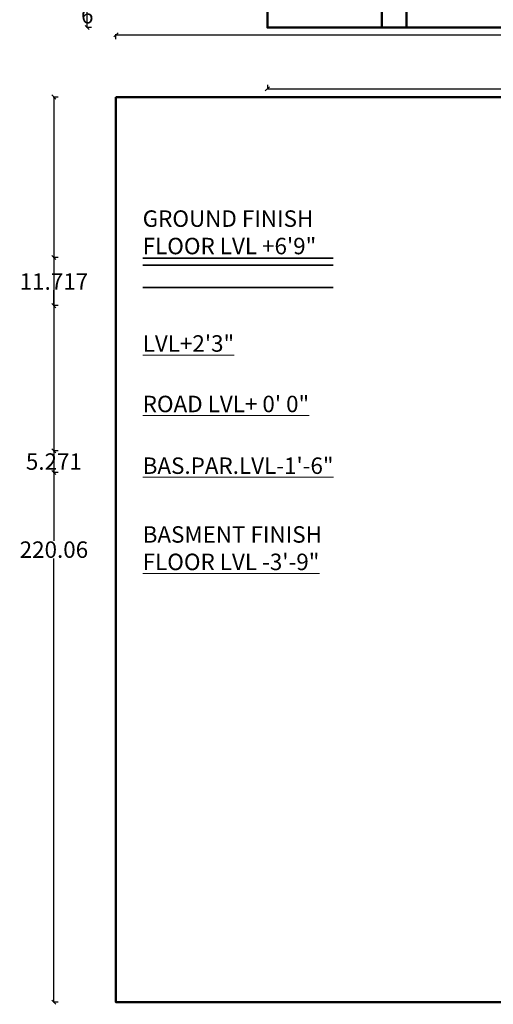
# Model space of a CAD drawing. Units: inches. Extents: x -60 to 284, y -245 to 257.
# Tile 1 of 10: x -60 to 55, y -228 to 12. Entities that reach past the tile are written whole.
import ezdxf

# ---------------------------------------------------------------- set-up
doc = ezdxf.new("R2010")
doc.units = ezdxf.units.IN
doc.header["$LTSCALE"] = 0.8
doc.header["$MEASUREMENT"] = 0
for name, color, linetype, lineweight in [('A-ANNO-DIMS', 2, 'Continuous', 18), ('A-ANNO-TEXT', 3, 'Continuous', 18), ('A-ANNO-TTLB', 7, 'Continuous', 50), ('A-SECT', 7, 'Continuous', 35), ('A-WALL', 7, 'Continuous', 50)]:
    doc.layers.add(name, color=color, linetype=linetype, lineweight=lineweight)
doc.styles.get("Standard").update_dxf_attribs({"font": 'arial.ttf'})
doc.dimstyles.get("Standard").update_dxf_attribs({"dimtxt": 4, "dimasz": 1, "dimexe": 0.18, "dimexo": 0.0625, "dimgap": 0.09, "dimtad": 0, "dimtih": 1, "dimtoh": 1, "dimzin": 0, "dimdsep": 46, "dimlunit": 4, "dimtxsty": 'Standard', "dimblk": 'OBLIQUE', "dimcen": 0.09, "dimadec": 0, "dimazin": 0, "dimtfac": 1, "dimtofl": 0, "dimtmove": 0, "dimatfit": 3, "dimfxl": 1, "dimfxlon": 1, "dimtolj": 1, "dimtzin": 0, "dimarcsym": 0})

# ---------------------------------------------------------------- blocks, each defined once
blk = doc.blocks.new('_Oblique')
at = {"color": 0, "linetype": 'ByBlock', "lineweight": -2}
blk.add_line((-0.5, -0.5), (0.5, 0.5), dxfattribs=at)
blk = doc.blocks.new('*D89')
at = {"layer": 'A-ANNO-DIMS', "color": 0, "lineweight": -2, "ltscale": 0.8, "transparency": 16777216}
for p, q in [((0.09, -4.23), (0.09, -5.41)), ((239.66, -4.23), (239.66, -5.41)), ((0.09, -5.23), (113, -5.23)), ((239.66, -5.23), (126.75, -5.23))]:
    blk.add_line(p, q, dxfattribs=at)
at = {"layer": 'Defpoints', "color": 0, "ltscale": 0.8, "transparency": 16777216}
for p in [(0.09, 9.67), (239.66, 9.67), (239.66, -5.23)]:
    blk.add_point(p, dxfattribs=at)
at = {"layer": 'A-ANNO-DIMS', "color": 0, "lineweight": -2, "ltscale": 0.8, "transparency": 16777216, "rotation": 180}
blk.add_blockref('_Oblique', (0.09, -5.23), dxfattribs=at)
at = {"layer": 'A-ANNO-DIMS', "color": 0, "lineweight": -2, "ltscale": 0.8, "transparency": 16777216}
blk.add_blockref('_Oblique', (239.66, -5.23), dxfattribs=at)
at = {"layer": 'A-ANNO-DIMS', "color": 0, "ltscale": 0.8, "transparency": 16777216, "insert": (119.88, -5.23), "char_height": 4, "attachment_point": 5}
blk.add_mtext('\\A1;239.6', dxfattribs=at)
blk = doc.blocks.new('*D90')
at = {"layer": 'A-ANNO-DIMS', "color": 0, "lineweight": -2, "ltscale": 0.8, "transparency": 16777216}
for p, q in [((-42.73, 122.67), (-43.91, 122.67)), ((-43.73, 122.67), (-43.73, 68.3)), ((-43.73, 9.67), (-43.73, 64.03)), ((-42.73, 9.67), (-43.91, 9.67))]:
    blk.add_line(p, q, dxfattribs=at)
at = {"layer": 'Defpoints', "color": 0, "ltscale": 0.8, "transparency": 16777216}
for p in [(-43.73, 122.67), (0.09, 122.67), (0.09, 9.67)]:
    blk.add_point(p, dxfattribs=at)
at = {"layer": 'A-ANNO-DIMS', "color": 0, "lineweight": -2, "ltscale": 0.8, "transparency": 16777216}
for p, rotation in [((-43.73, 122.67), 90), ((-43.73, 9.67), 270)]:
    blk.add_blockref('_Oblique', p, dxfattribs=dict(at, rotation=rotation))
at = {"layer": 'A-ANNO-DIMS', "color": 0, "ltscale": 0.8, "transparency": 16777216, "insert": (-43.73, 66.17), "char_height": 4, "attachment_point": 5}
blk.add_mtext('\\A1;113', dxfattribs=at)
blk = doc.blocks.new('*D101')
at = {"layer": 'A-ANNO-DIMS', "color": 0, "lineweight": -2, "ltscale": 0.8, "transparency": 16777216}
for p, q in [((-42.73, 15.67), (-43.91, 15.67)), ((-43.73, 15.67), (-43.73, 14.8)), ((-42.73, 9.67), (-43.91, 9.67)), ((-43.73, 9.67), (-43.73, 10.53))]:
    blk.add_line(p, q, dxfattribs=at)
at = {"layer": 'Defpoints', "color": 0, "ltscale": 0.8, "transparency": 16777216}
for p in [(-43.73, 15.67), (33.94, 15.67), (33.94, 9.67)]:
    blk.add_point(p, dxfattribs=at)
at = {"layer": 'A-ANNO-DIMS', "color": 0, "lineweight": -2, "ltscale": 0.8, "transparency": 16777216}
for p, rotation in [((-43.73, 15.67), 90), ((-43.73, 9.67), 270)]:
    blk.add_blockref('_Oblique', p, dxfattribs=dict(at, rotation=rotation))
at = {"layer": 'A-ANNO-DIMS', "color": 0, "ltscale": 0.8, "transparency": 16777216, "insert": (-43.73, 12.67), "char_height": 4, "attachment_point": 5}
blk.add_mtext('\\A1;6', dxfattribs=at)
blk = doc.blocks.new('*D106')
at = {"layer": 'A-ANNO-DIMS', "color": 0, "lineweight": -2, "ltscale": 0.8, "transparency": 16777216}
for p, q in [((-50.85, -93.21), (-52.03, -93.21)), ((-51.85, -93.21), (-51.85, -93.71)), ((-51.85, -98.48), (-51.85, -97.98)), ((-50.85, -98.48), (-52.03, -98.48))]:
    blk.add_line(p, q, dxfattribs=at)
at = {"layer": 'Defpoints', "color": 0, "ltscale": 0.8, "transparency": 16777216}
for p in [(67.01, -93.21), (-51.85, -98.48), (67.01, -98.48)]:
    blk.add_point(p, dxfattribs=at)
at = {"layer": 'A-ANNO-DIMS', "color": 0, "lineweight": -2, "ltscale": 0.8, "transparency": 16777216}
for p, rotation in [((-51.85, -93.21), 90), ((-51.85, -98.48), 270)]:
    blk.add_blockref('_Oblique', p, dxfattribs=dict(at, rotation=rotation))
at = {"layer": 'A-ANNO-DIMS', "color": 0, "ltscale": 0.8, "transparency": 16777216, "insert": (-51.85, -95.84), "char_height": 4, "attachment_point": 5}
blk.add_mtext('\\A1;5.271', dxfattribs=at)
blk = doc.blocks.new('*D111')
at = {"layer": 'A-ANNO-DIMS', "color": 0, "lineweight": -2, "ltscale": 0.8, "transparency": 16777216}
for p, q in [((-50.85, -46.21), (-52.03, -46.21)), ((-51.85, -46.21), (-51.85, -49.97)), ((-51.85, -57.93), (-51.85, -54.17)), ((-50.85, -57.93), (-52.03, -57.93))]:
    blk.add_line(p, q, dxfattribs=at)
at = {"layer": 'Defpoints', "color": 0, "ltscale": 0.8, "transparency": 16777216}
for p in [(193.74, -46.21), (-51.85, -57.93), (193.74, -57.93)]:
    blk.add_point(p, dxfattribs=at)
at = {"layer": 'A-ANNO-DIMS', "color": 0, "lineweight": -2, "ltscale": 0.8, "transparency": 16777216}
for p, rotation in [((-51.85, -46.21), 90), ((-51.85, -57.93), 270)]:
    blk.add_blockref('_Oblique', p, dxfattribs=dict(at, rotation=rotation))
at = {"layer": 'A-ANNO-DIMS', "color": 0, "ltscale": 0.8, "transparency": 16777216, "insert": (-51.85, -52.07), "char_height": 4, "attachment_point": 5}
blk.add_mtext('\\A1;11.717', dxfattribs=at)
blk = doc.blocks.new('*D114')
at = {"layer": 'A-ANNO-DIMS', "color": 0, "lineweight": -2, "ltscale": 0.8, "transparency": 16777216}
for p, q in [((-36.75, 6.88), (-36.75, 8.06)), ((-36.75, 7.88), (100.05, 7.88)), ((253.69, 7.88), (116.89, 7.88)), ((253.69, 6.88), (253.69, 8.06))]:
    blk.add_line(p, q, dxfattribs=at)
at = {"layer": 'Defpoints', "color": 0, "ltscale": 0.8, "transparency": 16777216}
for p in [(253.69, 7.88), (-36.75, -7.22), (253.69, -7.22)]:
    blk.add_point(p, dxfattribs=at)
at = {"layer": 'A-ANNO-DIMS', "color": 0, "lineweight": -2, "ltscale": 0.8, "transparency": 16777216, "rotation": 180}
blk.add_blockref('_Oblique', (-36.75, 7.88), dxfattribs=at)
at = {"layer": 'A-ANNO-DIMS', "color": 0, "lineweight": -2, "ltscale": 0.8, "transparency": 16777216}
blk.add_blockref('_Oblique', (253.69, 7.88), dxfattribs=at)
at = {"layer": 'A-ANNO-DIMS', "color": 0, "ltscale": 0.8, "transparency": 16777216, "insert": (108.47, 7.88), "char_height": 4, "attachment_point": 5}
blk.add_mtext('\\A1;290.44', dxfattribs=at)
blk = doc.blocks.new('*D115')
at = {"layer": 'A-ANNO-DIMS', "color": 0, "lineweight": -2, "ltscale": 0.8, "transparency": 16777216}
for p, q in [((-50.85, -7.22), (-52.03, -7.22)), ((-51.85, -7.22), (-51.85, -115.12)), ((-51.85, -227.28), (-51.85, -119.39)), ((-50.85, -227.28), (-52.03, -227.28))]:
    blk.add_line(p, q, dxfattribs=at)
at = {"layer": 'Defpoints', "color": 0, "ltscale": 0.8, "transparency": 16777216}
for p in [(-51.85, -7.22), (-36.75, -7.22), (-36.75, -227.28)]:
    blk.add_point(p, dxfattribs=at)
at = {"layer": 'A-ANNO-DIMS', "color": 0, "lineweight": -2, "ltscale": 0.8, "transparency": 16777216}
for p, rotation in [((-51.85, -7.22), 90), ((-51.85, -227.28), 270)]:
    blk.add_blockref('_Oblique', p, dxfattribs=dict(at, rotation=rotation))
at = {"layer": 'A-ANNO-DIMS', "color": 0, "ltscale": 0.8, "transparency": 16777216, "insert": (-51.85, -117.25), "char_height": 4, "attachment_point": 5}
blk.add_mtext('\\A1;220.06', dxfattribs=at)

msp = doc.modelspace()

# ---------------------------------------------------------------- linework, layer by layer
at = {"layer": 'A-ANNO-TTLB', "ltscale": 0.8}
for points in [[(0.0867, 122.666), (239.6639, 122.666), (239.6639, 9.666), (0.0867, 9.666)], [(-36.7489, -7.223), (253.6882, -7.223), (253.6882, -227.2835), (-36.7489, -227.2835)]]:
    msp.add_lwpolyline(points, close=True, dxfattribs=at)
at = {"layer": 'A-SECT', "ltscale": 0.8}
for p, q in [((-30.2246, -46.3771), (16.0973, -46.3771)), ((-30.2246, -48.0672), (16.0973, -48.0672)), ((-30.2246, -53.543), (16.0973, -53.543))]:
    msp.add_line(p, q, dxfattribs=at)
at = {"layer": 'A-WALL'}
for points in [[(198.9361, 9.666), (198.9361, 21.666), (159.9361, 21.666), (79.9361, 21.666), (37.9361, 21.666), (27.9361, 21.666), (27.9361, 9.666)], [(192.9361, 9.666), (192.9361, 15.666), (159.9361, 15.666), (79.9361, 15.666), (37.9361, 15.666), (33.9361, 15.666), (33.9361, 9.666)]]:
    msp.add_lwpolyline(points, dxfattribs=at)

# ---------------------------------------------------------------- texts
at = {"layer": 'A-ANNO-TEXT', "ltscale": 0.8, "char_height": 4, "attachment_point": 1}
for s, insert in [('{\\fArial|b1|i0|c0|p34;GROUND FINISH\\PFLOOR LVL +6\'9"}', (-30.2427, -34.7741)), ('{\\fArial|b1|i0|c0|p34;\\LLVL+2\'3"}', (-30.2427, -65.1324)), ('{\\fArial|b1|i0|c0|p34;\\LROAD LVL+ 0\' 0"}', (-30.2427, -79.8404)), ('{\\fArial|b1|i0|c0|p34;\\LBAS.PAR.LVL-1\'-6"}', (-30.2427, -94.8393)), ('{\\fArial|b1|i0|c0|p34;BASMENT FINISH\\P\\LFLOOR LVL -3\'-9"}', (-30.2427, -111.5594))]:
    msp.add_mtext_dynamic_manual_height_columns(s, width=97.551324, gutter_width=1, heights=[0], dxfattribs=dict(at, insert=insert))

# ---------------------------------------------------------------- dimensions: what is measured, and where the dimension line sits
at = {"layer": 'A-ANNO-DIMS', "ltscale": 0.8}
for base, p1, p2, override, picture, middle in [((-43.7318, 122.666), (0.0867, 9.666), (0.0867, 122.666), {"dimdec": 0, "dimlfac": 1, "dimrnd": 0, "dimzin": 0, "dimdsep": 46, "dimlunit": 2}, '*D90', (-43.7318, 66.166)), ((-43.7318, 15.666), (33.9361, 9.666), (33.9361, 15.666), {"dimdec": 0, "dimlfac": 1, "dimrnd": 0, "dimzin": 0, "dimdsep": 46, "dimlunit": 2}, '*D101', (-43.7318, 12.666)), ((-51.8489, -7.223), (-36.7489, -227.2835), (-36.7489, -7.223), {"dimdec": 2, "dimlfac": 1, "dimrnd": 0, "dimzin": 0, "dimdsep": 46, "dimlunit": 2}, '*D115', (-51.8489, -117.2532)), ((-51.8489, -57.9262), (193.7426, -46.2089), (193.7426, -57.9262), {"dimdec": 3, "dimlfac": 1, "dimrnd": 0, "dimzin": 0, "dimdsep": 46, "dimlunit": 2}, '*D111', (-51.8489, -52.0675)), ((-51.8489, -98.4801), (67.0139, -93.2089), (67.0139, -98.4801), {"dimdec": 3, "dimlfac": 1, "dimrnd": 0, "dimzin": 0, "dimdsep": 46, "dimlunit": 2}, '*D106', (-51.8489, -95.8445))]:
    dim = msp.add_linear_dim(base=base, p1=p1, p2=p2, angle=90, dimstyle='Standard', override=override, dxfattribs=at)
    dim.commit()
    dim.dimension.update_dxf_attribs({"geometry": picture, "text_midpoint": middle})
for base, p1, p2, override, picture, middle in [((253.6882, 7.877), (-36.7489, -7.223), (253.6882, -7.223), {"dimdec": 2, "dimlfac": 1, "dimrnd": 0, "dimzin": 0, "dimdsep": 46, "dimlunit": 2}, '*D114', (108.4697, 7.877)), ((239.6639, -5.234), (0.0867, 9.666), (239.6639, 9.666), {"dimdec": 1, "dimlfac": 1, "dimrnd": 0, "dimzin": 0, "dimdsep": 46, "dimlunit": 2}, '*D89', (119.8753, -5.234))]:
    dim = msp.add_linear_dim(base=base, p1=p1, p2=p2, dimstyle='Standard', override=override, dxfattribs=at)
    dim.commit()
    dim.dimension.update_dxf_attribs({"geometry": picture, "text_midpoint": middle})

doc.saveas('drawing.dxf')
